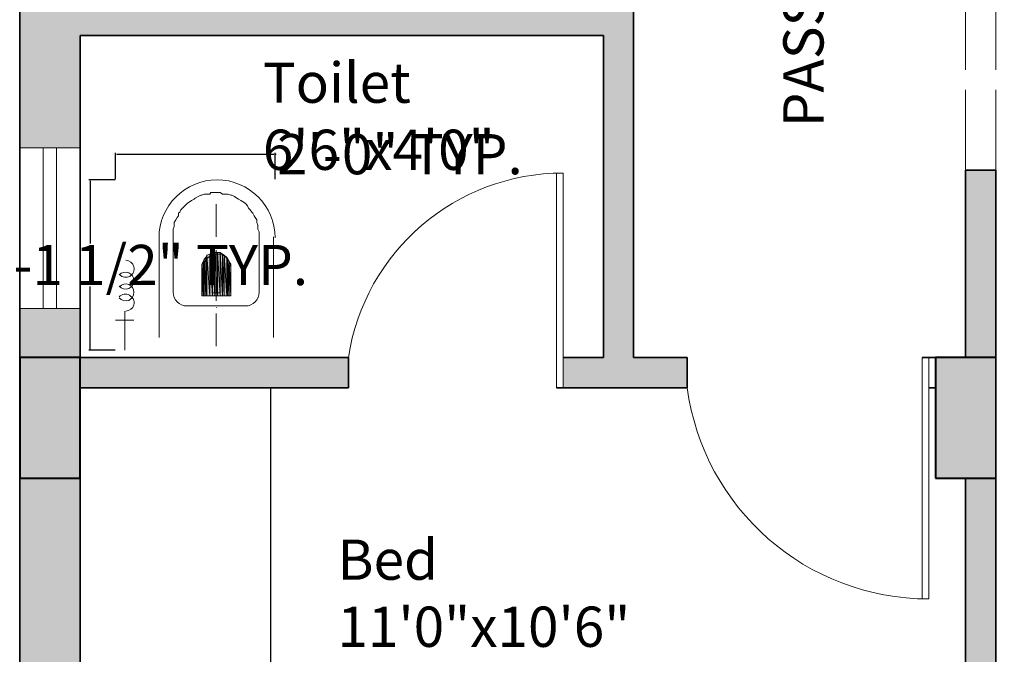
# Model space of a CAD drawing. Units: inches. Extents: x 56944 to 57417, y 173916 to 174454.
# Tile 3 of 8: x 57034 to 57181, y 174056 to 174150. Entities that reach past the tile are written whole.
import ezdxf

# ---------------------------------------------------------------- set-up
doc = ezdxf.new("R2010")
doc.units = ezdxf.units.IN
doc.header["$MEASUREMENT"] = 0
doc.linetypes.add('ACAD_ISO02W100', pattern=[15, 12, -3])
for name, color, linetype, lineweight in [('A-ANNO-DIMS', 2, 'Continuous', 18), ('A-AREA-IDEN', 7, 'Continuous', 20), ('A-COLS', 7, 'Continuous', 40), ('A-COLS-PATT', 250, 'Continuous', 9), ('A-DOOR', 3, 'Continuous', 20), ('A-FLOR-CASE', 8, 'Continuous', 25), ('A-FLOR-FIXT', 9, 'Continuous', 18), ('A-GLAZ', 4, 'Continuous', 18), ('A-SITE-PATT', 8, 'Continuous', 9), ('A-WALL', 7, 'Continuous', 35), ('A-WALL-OVHD', 7, 'ACAD_ISO02W100', 18), ('A-WALL-PATT', 241, 'Continuous', 9)]:
    doc.layers.add(name, color=color, linetype=linetype, lineweight=lineweight)
doc.styles.get("Standard").update_dxf_attribs({"font": 'arial.ttf'})
doc.dimstyles.get("Standard").update_dxf_attribs({"dimtxt": 6, "dimasz": 0.18, "dimexe": 0.18, "dimexo": 0.0625, "dimgap": 0.09, "dimtad": 0, "dimtih": 1, "dimtoh": 1, "dimdec": 1, "dimzin": 0, "dimdsep": 46, "dimlunit": 3, "dimtxsty": 'Standard', "dimcen": 0.09, "dimadec": 0, "dimazin": 0, "dimtfac": 1, "dimtdec": 1, "dimtofl": 0, "dimtmove": 0, "dimatfit": 3, "dimfxl": 1, "dimtolj": 1, "dimtzin": 0, "dimarcsym": 0})

# ---------------------------------------------------------------- blocks, each defined once
blk = doc.blocks.new('WC-PLAN')
h = blk.add_hatch(color=256)
h.paths.add_polyline_path([(13.07, 8.12), (13.07, 13.2), (13.22, 8.12)])
h.paths.add_polyline_path([(13.07, 13.2), (13.22, 8.12), (13.22, 13.58)])
h = blk.add_hatch(color=256)
h.paths.add_polyline_path([(13.22, 8.12), (13.22, 13.58), (13.45, 8.12)])
h.paths.add_polyline_path([(13.22, 13.58), (13.45, 8.12), (13.45, 13.81)])
h = blk.add_hatch(color=256)
h.paths.add_polyline_path([(13.45, 8.12), (13.45, 13.81), (13.6, 8.12)])
h.paths.add_polyline_path([(13.45, 13.81), (13.6, 8.12), (13.6, 14.19)])
h = blk.add_hatch(color=256)
h.paths.add_polyline_path([(13.6, 8.12), (13.6, 14.19), (14.06, 8.12)])
h.paths.add_polyline_path([(13.6, 14.19), (14.06, 8.12), (14.06, 14.34)])
h = blk.add_hatch(color=256)
h.paths.add_polyline_path([(14.06, 8.12), (14.06, 14.34), (14.44, 8.12)])
h.paths.add_polyline_path([(14.06, 14.34), (14.44, 8.12), (14.44, 14.56)])
h = blk.add_hatch(color=256)
h.paths.add_polyline_path([(14.44, 8.12), (14.44, 14.56), (14.81, 8.12)])
h.paths.add_polyline_path([(14.44, 14.56), (14.81, 8.12), (14.81, 14.56)])
h = blk.add_hatch(color=256)
h.paths.add_polyline_path([(14.81, 8.12), (14.81, 14.56), (15.19, 8.12)])
h.paths.add_polyline_path([(14.81, 14.56), (15.19, 8.12), (15.19, 14.56)])
h = blk.add_hatch(color=256)
h.paths.add_polyline_path([(15.19, 8.12), (15.19, 14.56), (15.57, 8.12)])
h.paths.add_polyline_path([(15.19, 14.56), (15.57, 8.12), (15.57, 14.56)])
h = blk.add_hatch(color=256)
h.paths.add_polyline_path([(15.57, 8.12), (15.57, 14.56), (15.95, 8.12)])
h.paths.add_polyline_path([(15.57, 14.56), (15.95, 8.12), (15.95, 14.34)])
h = blk.add_hatch(color=256)
h.paths.add_polyline_path([(15.95, 8.12), (15.95, 14.34), (16.18, 8.12)])
h.paths.add_polyline_path([(15.95, 14.34), (16.18, 8.12), (16.18, 14.19)])
h = blk.add_hatch(color=256)
h.paths.add_polyline_path([(16.18, 8.12), (16.18, 14.19), (16.56, 8.12)])
h.paths.add_polyline_path([(16.18, 14.19), (16.56, 8.12), (16.56, 13.81)])
h = blk.add_hatch(color=256)
h.paths.add_polyline_path([(16.56, 8.12), (16.56, 13.81), (16.71, 8.12)])
h.paths.add_polyline_path([(16.56, 13.81), (16.71, 8.12), (16.71, 13.58)])
h = blk.add_hatch(color=256)
h.paths.add_polyline_path([(16.71, 8.12), (16.71, 13.58), (16.94, 8.12)])
h.paths.add_polyline_path([(16.71, 13.58), (16.94, 8.12), (16.94, 13.2)])
h = blk.add_hatch(color=256)
h.paths.add_polyline_path([(12.84, 8.12), (12.84, 12.82), (13.07, 8.12)])
h.paths.add_polyline_path([(12.84, 12.82), (13.07, 8.12), (13.07, 13.2)])
h = blk.add_hatch(color=256)
h.paths.add_polyline_path([(16.94, 8.12), (16.94, 13.2), (17.17, 8.12)])
h.paths.add_polyline_path([(16.94, 13.2), (17.17, 8.12), (17.17, 12.82)])
h.paths.add_polyline_path([(17.17, 8.12), (17.17, 12.82), (17.17, 12.44)])
for points in [[(21.41, 15.93), (21.41, 16.69), (21.41, 17.3), (21.41, 17.67), (21.19, 18.05), (21.19, 18.43), (21.19, 18.66), (21.03, 19.04), (21.03, 19.42), (20.81, 19.8), (20.66, 20.03), (20.43, 20.41), (20.28, 20.56), (20.05, 20.94), (19.82, 21.16), (19.67, 21.54), (19.44, 21.77), (19.29, 21.92), (18.91, 22.15), (18.68, 22.3), (18.3, 22.53), (18.08, 22.68), (17.7, 22.91), (17.32, 23.14), (17.17, 23.14), (16.71, 23.29), (16.33, 23.29), (15.95, 23.29), (15.57, 23.52), (14.97, 23.52), (14.21, 23.52), (14.06, 23.29), (13.6, 23.29), (13.22, 23.29), (12.84, 23.14), (12.69, 23.14), (12.31, 22.91), (11.86, 22.68), (11.7, 22.53), (11.32, 22.3), (11.1, 22.15), (10.72, 21.92), (10.57, 21.77), (10.34, 21.54), (9.96, 21.16), (9.73, 20.94), (9.58, 20.56), (9.35, 20.41), (9.35, 20.03), (9.2, 19.8), (8.97, 19.42), (8.75, 19.04), (8.75, 18.66), (8.75, 18.43), (8.59, 18.05), (8.59, 17.67), (8.59, 17.3), (8.59, 16.69), (8.59, 15.93)], [(14.97, 16.92), (14.97, 21.77), (14.97, 21.77)], [(6.47, 1.9), (6.47, 16.92), (6.47, 16.92)], [(23.54, 1.9), (23.54, 16.92), (23.54, 16.92)], [(8.59, 8.72), (8.59, 15.93), (8.59, 15.93)], [(14.97, 7.36), (14.97, 14.94), (14.97, 14.94)], [(21.41, 8.72), (21.41, 15.93), (21.41, 15.93)], [(12.84, 8.12), (12.84, 12.44), (12.84, 12.44)], [(17.17, 8.12), (17.17, 12.44), (17.17, 12.44)], [(17.17, 8.12), (12.84, 8.12), (12.84, 8.12)], [(14.59, 8.57), (14.59, 8.5), (14.59, 8.5)], [(14.97, 8.57), (14.81, 8.57), (14.59, 8.57)], [(14.97, 8.57), (15.04, 8.5), (15.04, 8.5)], [(15.42, 8.57), (15.19, 8.57), (14.97, 8.57)], [(15.42, 8.57), (15.42, 8.5), (15.42, 8.5)], [(19.29, 6.6), (10.57, 6.6), (10.57, 6.6)], [(14.97, 6.37), (15.04, 6.37), (15.04, 6.37)], [(2.73, 4.48), (0, 4.48), (0, 4.48)], [(1.37, 0), (1.37, 5.84), (1.37, 5.84)], [(14.97, 0.61), (14.97, 5.46), (14.97, 5.46)]]:
    blk.add_lwpolyline(points)
for points in [[(13.07, 13.2), (13.22, 8.12), (13.22, 13.58)], [(13.22, 13.58), (13.45, 8.12), (13.45, 13.81)], [(13.22, 8.12), (13.22, 13.58), (13.45, 8.12)], [(13.45, 13.81), (13.6, 8.12), (13.6, 14.19)], [(13.45, 8.12), (13.45, 13.81), (13.6, 8.12)], [(13.6, 14.19), (14.06, 8.12), (14.06, 14.34)], [(13.6, 8.12), (13.6, 14.19), (14.06, 8.12)], [(14.06, 14.34), (14.44, 8.12), (14.44, 14.56)], [(14.06, 8.12), (14.06, 14.34), (14.44, 8.12)], [(14.44, 8.12), (14.44, 14.56), (14.81, 8.12)], [(14.44, 14.56), (14.81, 8.12), (14.81, 14.56)], [(14.81, 8.12), (14.81, 14.56), (15.19, 8.12)], [(14.81, 14.56), (15.19, 8.12), (15.19, 14.56)], [(15.19, 8.12), (15.19, 14.56), (15.57, 8.12)], [(15.19, 14.56), (15.57, 8.12), (15.57, 14.56)], [(15.57, 8.12), (15.57, 14.56), (15.95, 8.12)], [(15.57, 14.56), (15.95, 8.12), (15.95, 14.34)], [(15.95, 8.12), (15.95, 14.34), (16.18, 8.12)], [(15.95, 14.34), (16.18, 8.12), (16.18, 14.19)], [(16.18, 8.12), (16.18, 14.19), (16.56, 8.12)], [(16.18, 14.19), (16.56, 8.12), (16.56, 13.81)], [(16.56, 8.12), (16.56, 13.81), (16.71, 8.12)], [(16.56, 13.81), (16.71, 8.12), (16.71, 13.58)], [(16.71, 8.12), (16.71, 13.58), (16.94, 8.12)], [(16.71, 13.58), (16.94, 8.12), (16.94, 13.2)], [(12.84, 12.82), (13.07, 8.12), (13.07, 13.2)], [(12.84, 12.44), (12.84, 8.12), (12.84, 12.82)], [(12.84, 8.12), (12.84, 12.82), (13.07, 8.12)], [(12.84, 8.12), (12.84, 12.44)], [(13.07, 8.12), (13.07, 13.2), (13.22, 8.12)], [(16.94, 8.12), (16.94, 13.2), (17.17, 8.12)], [(16.94, 13.2), (17.17, 8.12), (17.17, 12.82)], [(17.17, 8.12), (17.17, 12.82), (17.17, 12.44)], [(17.17, 12.82), (17.17, 8.12), (17.17, 8.12)]]:
    blk.add_lwpolyline(points, close=True)
for points, knots in [([(6.47, 16.76), (6.47, 21.54), (10.34, 25.41), (15.12, 25.41), (15.12, 25.41), (19.9, 25.41), (23.77, 21.54), (23.77, 16.76)], [0, 0, 0, 0, 0.125, 0.125, 0.125, 0.125001, 1, 1, 1, 1]), ([(1.52, 13.43), (2.05, 13.43), (2.58, 12.97), (2.73, 12.44), (2.73, 12.44), (2.88, 11.91), (2.58, 11.3), (2.12, 11), (2.12, 11), (1.59, 10.77), (0.99, 10.85), (0.61, 11.23)], [0, 0, 0, 0, 0.083333, 0.083333, 0.083333, 0.083334, 0.166667, 0.166667, 0.166667, 0.166668, 1, 1, 1, 1]), ([(13.07, 12.29), (13.07, 13.43), (13.98, 14.34), (15.12, 14.34), (15.12, 14.34), (16.26, 14.34), (17.17, 13.43), (17.17, 12.29)], [0, 0, 0, 0, 0.125, 0.125, 0.125, 0.125001, 1, 1, 1, 1]), ([(0.53, 11.23), (0.91, 11.61), (1.44, 11.76), (1.97, 11.53), (1.97, 11.53), (2.43, 11.38), (2.73, 10.92), (2.73, 10.39), (2.73, 10.39), (2.73, 9.86), (2.43, 9.41), (1.97, 9.18), (1.97, 9.18), (1.44, 9.03), (0.91, 9.18), (0.53, 9.56)], [0, 0, 0, 0, 0.0625, 0.0625, 0.0625, 0.062501, 0.125, 0.125, 0.125, 0.125001, 0.1875, 0.1875, 0.1875, 0.187501, 1, 1, 1, 1]), ([(0.61, 9.48), (0.91, 9.86), (1.52, 10.01), (1.97, 9.79), (1.97, 9.79), (2.43, 9.63), (2.73, 9.1), (2.73, 8.65), (2.73, 8.65), (2.73, 8.12), (2.43, 7.66), (1.97, 7.43), (1.97, 7.43), (1.44, 7.28), (0.91, 7.43), (0.53, 7.81)], [0, 0, 0, 0, 0.0625, 0.0625, 0.0625, 0.062501, 0.125, 0.125, 0.125, 0.125001, 0.1875, 0.1875, 0.1875, 0.187501, 1, 1, 1, 1]), ([(0.53, 7.97), (0.91, 8.34), (1.59, 8.5), (2.05, 8.19), (2.05, 8.19), (2.58, 7.89), (2.88, 7.36), (2.73, 6.75), (2.73, 6.75), (2.58, 6.22), (2.05, 5.84), (1.52, 5.84)], [0, 0, 0, 0, 0.083333, 0.083333, 0.083333, 0.083334, 0.166667, 0.166667, 0.166667, 0.166668, 1, 1, 1, 1])]:
    blk.add_open_spline(points, degree=3, knots=knots)
for points in [[(10.64, 6.6), (9.5, 6.6), (8.59, 7.51), (8.59, 8.65)], [(21.41, 8.65), (21.41, 7.51), (20.5, 6.6), (19.37, 6.6)]]:
    blk.add_open_spline(points, degree=3)
blk = doc.blocks.new('DOOR-SINGLE-36IN')
for p, q in [((35, 36), (35, 0)), ((36, 0), (36, 36)), ((36, 36), (36, 0)), ((36, 0), (35, 0))]:
    blk.add_line(p, q)
blk.add_arc((36, -0.32), 36.32, 90, 172.3719)
blk = doc.blocks.new('DOOR-SINGLE-32IN')
for p, q in [((32, 32), (31, 32)), ((31, 0), (31, 32)), ((32, 32), (32, 0))]:
    blk.add_line(p, q)
blk.add_arc((32, 32.37), 32.37, 188.6501, 270)
blk = doc.blocks.new('*D20')
at = {"layer": 'A-ANNO-DIMS', "color": 0, "lineweight": -2, "transparency": 16777216}
for p, q in [((57048.37, 174126.33), (57044.44, 174126.33)), ((57044.62, 174126.15), (57044.62, 174116.81)), ((57044.62, 174101.09), (57044.62, 174110.43)), ((57048.37, 174100.91), (57044.44, 174100.91))]:
    blk.add_line(p, q, dxfattribs=at)
at = {"layer": 'A-ANNO-DIMS', "color": 0, "transparency": 16777216}
for points in [[(57044.59, 174126.15), (57044.65, 174126.15), (57044.62, 174126.33)], [(57044.59, 174101.09), (57044.65, 174101.09), (57044.62, 174100.91)]]:
    blk.add_solid(points, dxfattribs=at)
at = {"layer": 'Defpoints', "color": 0, "transparency": 16777216}
for p in [(57044.62, 174126.33), (57048.43, 174126.33), (57048.43, 174100.91)]:
    blk.add_point(p, dxfattribs=at)
at = {"layer": 'A-ANNO-DIMS', "color": 0, "transparency": 16777216, "insert": (57044.62, 174113.62), "char_height": 6, "attachment_point": 5}
blk.add_mtext('\\A1;WC 2\'-1 1/2" TYP.', dxfattribs=at)
blk = doc.blocks.new('*D21')
at = {"layer": 'A-ANNO-DIMS', "color": 0, "lineweight": -2, "transparency": 16777216}
for p, q in [((57048.43, 174126.39), (57048.43, 174130.32)), ((57048.61, 174130.14), (57072.02, 174130.14)), ((57072.2, 174126.39), (57072.2, 174130.32)), ((57072.2, 174130.14), (57072.38, 174130.14))]:
    blk.add_line(p, q, dxfattribs=at)
at = {"layer": 'A-ANNO-DIMS', "color": 0, "transparency": 16777216}
for points in [[(57048.61, 174130.17), (57048.61, 174130.11), (57048.43, 174130.14)], [(57072.02, 174130.17), (57072.02, 174130.11), (57072.2, 174130.14)]]:
    blk.add_solid(points, dxfattribs=at)
at = {"layer": 'Defpoints', "color": 0, "transparency": 16777216}
for p in [(57072.2, 174130.14), (57048.43, 174126.33), (57072.2, 174126.33)]:
    blk.add_point(p, dxfattribs=at)
at = {"layer": 'A-ANNO-DIMS', "color": 0, "transparency": 16777216, "insert": (57090.81, 174130.14), "char_height": 6, "attachment_point": 5}
blk.add_mtext('\\A1;2\'-0" TYP.', dxfattribs=at)

msp = doc.modelspace()

# ---------------------------------------------------------------- hatches: boundary and pattern name
at = {"layer": 'A-COLS-PATT'}
h = msp.add_hatch(color=256, dxfattribs=at)
h.dxf.hatch_style = 1
h.paths.add_polyline_path([(57052.13, 174321.82), (57034.13, 174321.82), (57034.13, 174312.82), (57052.13, 174312.82)])
h.paths.add_polyline_path([(57186.38, 174321.82), (57168.38, 174321.82), (57168.38, 174312.82), (57175.13, 174312.82), (57186.38, 174312.82)])
h.paths.add_polyline_path([(57308.63, 174321.82), (57290.63, 174321.82), (57290.63, 174312.82), (57308.63, 174312.82)])
h.paths.add_polyline_path([(57179.63, 174204.82), (57170.63, 174204.82), (57170.63, 174186.82), (57179.63, 174186.82)])
h.paths.add_polyline_path([(57043.13, 174204.82), (57034.13, 174204.82), (57034.13, 174186.82), (57043.13, 174186.82)])
h.paths.add_polyline_path([(57308.63, 174206.32), (57299.63, 174206.32), (57299.63, 174188.32), (57308.63, 174188.32)])
h.paths.add_polyline_path([(57308.63, 174107.87), (57299.63, 174107.87), (57299.63, 174093.93), (57308.63, 174093.93)])
h.paths.add_polyline_path([(57308.63, 173978.32), (57299.63, 173978.32), (57299.63, 173960.32), (57308.63, 173960.32)])
h.paths.add_polyline_path([(57179.63, 173969.32), (57161.63, 173969.32), (57161.63, 173960.32), (57179.63, 173960.32)])
h.paths.add_polyline_path([(57043.13, 173978.32), (57034.13, 173978.32), (57034.13, 173960.32), (57043.13, 173960.32)])
h.paths.add_polyline_path([(57043.13, 174099.82), (57034.13, 174099.82), (57034.13, 174081.82), (57043.13, 174081.82)])
h.paths.add_polyline_path([(57179.63, 174099.82), (57170.63, 174099.82), (57170.63, 174081.82), (57179.63, 174081.82)])
at = {"layer": 'A-SITE-PATT'}
h = msp.add_hatch(dxfattribs=at)
h.set_pattern_fill('ANGLE', color=256, scale=50)
h.set_pattern_definition([(0, (0, 0), (0, 13.75), [10, -3.75]), (90, (0, 0), (-13.75, 8e-16), [10, -3.75])])
h.paths.add_polyline_path([(57365.63, 174396.82), (57200.13, 174396.82), (57200.13, 174379.18), (57215.46, 174379.18, -1.049383), (57218.84, 174379.34, -0.952941), (57215.46, 174379.18), (57200.13, 174379.18), (57200.13, 174360.82), (57140.13, 174360.82), (57140.13, 174321.82), (57149.42, 174321.82), (57243.2, 174321.82), (57282.32, 174321.82), (57283.32, 174321.82), (57308.63, 174321.82), (57308.63, 174305.82), (57308.63, 174259.72), (57308.63, 174258.72), (57308.63, 174252.72), (57308.63, 174216.72), (57308.63, 174099.82), (57308.63, 174093.93), (57308.63, 174081.93), (57308.63, 173969.32), (57365.63, 173969.32)])
h.paths.add_polyline_path([(57341.88, 174114.38), (57341.88, 174209.81), (57329.51, 174209.81), (57329.51, 174114.38)], flags=24)
h.paths.add_polyline_path([(57215.63, 174350.61), (57326.6, 174350.61), (57326.6, 174362.97), (57215.63, 174362.97)], flags=24)
at = {"layer": 'A-WALL-PATT'}
h = msp.add_hatch(color=256, dxfattribs=at)
h.dxf.hatch_style = 1
h.paths.add_polyline_path([(57089.42, 174321.82), (57052.13, 174321.82), (57052.13, 174312.82), (57089.42, 174312.82)])
h.paths.add_polyline_path([(57168.38, 174321.82), (57149.42, 174321.82), (57149.42, 174312.82), (57168.38, 174312.82)])
h.paths.add_polyline_path([(57199.66, 174321.82), (57186.38, 174321.82), (57186.38, 174312.82), (57199.66, 174312.82)])
h.paths.add_polyline_path([(57179.63, 174312.82), (57177.38, 174312.82), (57175.13, 174312.82), (57175.13, 174204.82), (57179.63, 174204.82)])
h.paths.add_polyline_path([(57043.13, 174312.82), (57034.13, 174312.82), (57034.13, 174204.82), (57043.13, 174204.82)])
h.paths.add_polyline_path([(57043.13, 174147.82), (57121.13, 174147.82), (57121.13, 174099.82), (57115.13, 174099.82), (57115.13, 174095.32), (57121.13, 174095.32), (57133.63, 174095.32), (57133.63, 174099.82), (57125.63, 174099.82), (57125.63, 174200.32), (57133.63, 174200.32), (57133.63, 174204.82), (57115.13, 174204.82), (57115.13, 174200.32), (57121.13, 174200.32), (57121.13, 174152.32), (57043.13, 174152.32), (57043.13, 174162.82), (57034.13, 174162.82), (57034.13, 174131.11), (57043.13, 174131.11)])
h.paths.add_polyline_path([(57043.13, 174081.82), (57034.13, 174081.82), (57034.13, 173978.32), (57043.13, 173978.32)])
h.paths.add_polyline_path([(57093.93, 173969.32), (57043.13, 173969.32), (57043.13, 173960.32), (57093.93, 173960.32)])
h.paths.add_polyline_path([(57161.63, 173969.32), (57153.93, 173969.32), (57153.93, 173960.32), (57161.63, 173960.32)])
h.paths.add_polyline_path([(57179.63, 174081.82), (57175.13, 174081.82), (57175.13, 173969.32), (57179.63, 173969.32)])
h.paths.add_polyline_path([(57299.63, 173969.32), (57179.63, 173969.32), (57179.63, 173960.32), (57299.63, 173960.32)])
h.paths.add_polyline_path([(57308.63, 174025.05), (57299.63, 174025.05), (57299.63, 173978.32), (57308.63, 173978.32)])
h.paths.add_polyline_path([(57308.63, 174081.93), (57299.63, 174081.93), (57299.63, 174075.82), (57227.63, 174075.82), (57227.63, 174081.82), (57223.13, 174081.82), (57223.13, 174075.82), (57223.13, 174071.32), (57299.63, 174071.32), (57299.63, 174061.05), (57308.63, 174061.05)])
h.paths.add_polyline_path([(57308.63, 174140.51), (57299.63, 174140.51), (57299.63, 174128.32), (57223.13, 174128.32), (57223.13, 174117.82), (57227.63, 174117.82), (57227.63, 174123.82), (57299.63, 174123.82), (57299.63, 174119.87), (57308.63, 174119.87)])
h.paths.add_polyline_path([(57308.63, 174216.72), (57299.63, 174216.72), (57299.63, 174206.32), (57308.63, 174206.32)])
h.paths.add_polyline_path([(57308.63, 174188.32), (57299.63, 174188.32), (57299.63, 174176.51), (57308.63, 174176.51)])
h.paths.add_polyline_path([(57308.63, 174258.72), (57299.63, 174258.72), (57299.63, 174252.72), (57308.63, 174252.72)])
h.paths.add_polyline_path([(57308.63, 174312.82), (57299.63, 174312.82), (57299.63, 174306.82), (57308.63, 174306.82)])
h.paths.add_polyline_path([(57290.63, 174321.82), (57283.32, 174321.82), (57283.32, 174312.82), (57290.63, 174312.82)])
h.paths.add_polyline_path([(57242.2, 174321.82), (57235.66, 174321.82), (57235.66, 174312.82), (57242.2, 174312.82)])
h.paths.add_polyline_path([(57083.13, 174204.82), (57043.13, 174204.82), (57043.13, 174200.32), (57083.13, 174200.32)], flags=17)
h.paths.add_polyline_path([(57083.13, 174099.82), (57043.13, 174099.82), (57043.13, 174095.32), (57083.13, 174095.32)], flags=0)
h = msp.add_hatch(color=256, dxfattribs=at)
h.dxf.hatch_style = 1
h.paths.add_polyline_path([(57043.13, 174107.11), (57034.13, 174107.11), (57034.13, 174099.82), (57043.13, 174099.82)])
h.paths.add_polyline_path([(57083.13, 174099.82), (57043.13, 174099.82), (57043.13, 174095.32), (57083.13, 174095.32)])
h.paths.add_polyline_path([(57179.63, 174127.74), (57175.13, 174127.74), (57175.13, 174099.82), (57179.63, 174099.82)])

# ---------------------------------------------------------------- linework, layer by layer
at = {"layer": 'A-COLS'}
for p, q in [((57034.13, 174099.82), (57034.13, 174081.82)), ((57043.13, 174099.82), (57034.13, 174099.82)), ((57043.13, 174081.82), (57043.13, 174099.82)), ((57179.63, 174099.82), (57170.63, 174099.82)), ((57170.63, 174099.82), (57170.63, 174081.82)), ((57034.13, 174081.82), (57043.13, 174081.82)), ((57170.63, 174081.82), (57179.63, 174081.82))]:
    msp.add_line(p, q, dxfattribs=at)
at = {"layer": 'A-DOOR'}
msp.add_line((57115.13, 174127.32), (57115.13, 174095.32), dxfattribs=at)
at = {"layer": 'A-FLOR-CASE'}
msp.add_line((57071.54, 174095.32), (57071.54, 173969.32), dxfattribs=at)
at = {"layer": 'A-GLAZ'}
for p, q in [((57043.13, 174131.11), (57034.13, 174131.11)), ((57034.13, 174131.11), (57034.13, 174107.11)), ((57037.63, 174131.11), (57037.63, 174107.11)), ((57039.63, 174107.11), (57039.63, 174131.11)), ((57043.13, 174107.11), (57043.13, 174131.11)), ((57034.13, 174107.11), (57043.13, 174107.11))]:
    msp.add_line(p, q, dxfattribs=at)
at = {"layer": 'A-WALL'}
for p, q in [((57034.13, 174321.82), (57034.13, 173960.32)), ((57125.63, 174200.32), (57125.63, 174099.82)), ((57043.13, 174147.82), (57121.13, 174147.82)), ((57043.13, 174147.82), (57043.13, 173960.32)), ((57121.13, 174147.82), (57121.13, 174099.82)), ((57175.13, 174127.74), (57175.13, 174099.82)), ((57175.13, 174127.74), (57179.63, 174127.74)), ((57179.63, 174127.74), (57179.63, 174099.82)), ((57034.13, 174099.82), (57083.13, 174099.82)), ((57083.13, 174095.32), (57083.13, 174099.82)), ((57115.13, 174099.82), (57121.13, 174099.82)), ((57125.63, 174099.82), (57133.63, 174099.82)), ((57133.63, 174099.82), (57133.63, 174095.32)), ((57168.63, 174099.82), (57179.63, 174099.82)), ((57170.63, 174099.82), (57169.63, 174099.82)), ((57179.63, 174099.82), (57179.63, 173960.32)), ((57043.13, 174095.32), (57083.13, 174095.32)), ((57114.13, 174095.32), (57133.63, 174095.32)), ((57121.13, 174095.32), (57115.13, 174095.32)), ((57169.63, 174095.32), (57170.63, 174095.32)), ((57175.13, 174081.82), (57175.13, 173969.32))]:
    msp.add_line(p, q, dxfattribs=at)
at = {"layer": 'A-WALL-OVHD'}
for p, q in [((57175.13, 174127.74), (57175.13, 174186.82)), ((57179.63, 174127.74), (57179.63, 174186.82))]:
    msp.add_line(p, q, dxfattribs=at)

# ---------------------------------------------------------------- block references
at = {"layer": 'A-DOOR', "extrusion": (0, 0, -1), "zscale": -1, "rotation": 180}
for name, p in [('DOOR-SINGLE-32IN', (-57083.13, 174127.32)), ('DOOR-SINGLE-36IN', (-57133.63, 174099.82))]:
    msp.add_blockref(name, p, dxfattribs=at)
at = {"layer": 'A-FLOR-FIXT'}
msp.add_blockref('WC-PLAN', (57048.43, 174100.91), dxfattribs=at)

# ---------------------------------------------------------------- texts
at = {"layer": 'A-AREA-IDEN', "insert": (57147.95, 174134.15), "char_height": 6, "attachment_point": 1, "rotation": 90}
msp.add_mtext_dynamic_manual_height_columns('PASSAGE', width=38.9548, gutter_width=1, heights=[0], dxfattribs=at)
at = {"layer": 'A-AREA-IDEN', "char_height": 6, "attachment_point": 1}
for s, width, insert in [('Toilet\\P6\'6"x4\'0"', 44.3012, (57070.37, 174143.8)), ('Bed\\P11\'0"x10\'6"', 61.1834, (57081.5, 174072.68))]:
    msp.add_mtext_dynamic_manual_height_columns(s, width=width, gutter_width=1, heights=[0], dxfattribs=dict(at, insert=insert))

# ---------------------------------------------------------------- dimensions: what is measured, and where the dimension line sits
at = {"layer": 'A-ANNO-DIMS'}
dim = msp.add_linear_dim(base=(57072.2, 174130.14), p1=(57048.43, 174126.33), p2=(57072.2, 174126.33), text='<> TYP.', dimstyle='Standard', override={"dimdec": 1, "dimlfac": 1, "dimrnd": 0, "dimzin": 1, "dimdsep": 46, "dimlunit": 4, "dimfrac": 2}, dxfattribs=at)
dim.commit()
dim.dimension.update_dxf_attribs({"geometry": '*D21', "text_midpoint": (57090.81, 174130.14)})
dim = msp.add_linear_dim(base=(57044.62, 174126.33), p1=(57048.43, 174100.91), p2=(57048.43, 174126.33), angle=90, text='WC <> TYP.', dimstyle='Standard', override={"dimdec": 1, "dimlfac": 1, "dimrnd": 0, "dimzin": 1, "dimdsep": 46, "dimlunit": 4, "dimfrac": 2}, dxfattribs=at)
dim.commit()
dim.dimension.update_dxf_attribs({"geometry": '*D20', "text_midpoint": (57044.62, 174113.62)})

doc.saveas('drawing.dxf')
